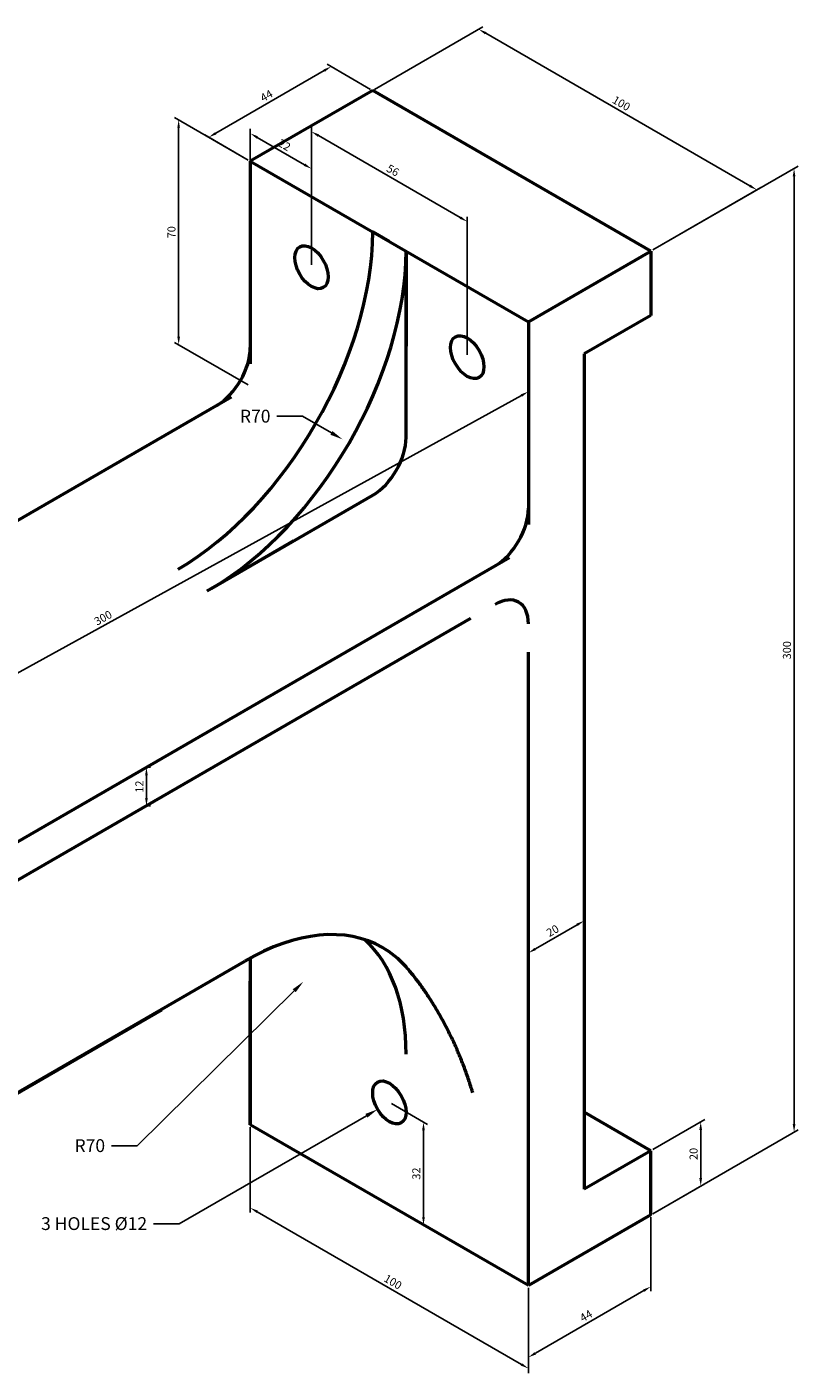
# Model space of a CAD drawing. Units: millimetres. Extents: x 3560 to 4017, y 1013 to 1432.
# Tile 2 of 2: x 3777 to 4017, y 1013 to 1432. Entities that reach past the tile are written whole.
import ezdxf
from ezdxf import colors
from ezdxf.entities.mleader import LeaderData, LeaderLine
from ezdxf.math import Vec2, Vec3

# ---------------------------------------------------------------- set-up
doc = ezdxf.new("R2010")
doc.units = ezdxf.units.MM
for name, color, linetype, lineweight in [('M-DIMS', 2, 'Continuous', 25), ('M-OUTL', 7, 'Continuous', 50), ('M-TEXT', 3, 'Continuous', 25)]:
    doc.layers.add(name, color=color, linetype=linetype, lineweight=lineweight)
doc.styles.get("Standard").update_dxf_attribs({"font": 'arial.ttf'})
doc.dimstyles.new('ISO-25', dxfattribs={"dimtxt": 2.5, "dimasz": 2.5, "dimexe": 1.25, "dimexo": 0.625, "dimtad": 1, "dimtxsty": 'Standard', "dimcen": 2.5, "dimadec": 0, "dimazin": 0, "dimtfac": 1, "dimtmove": 0, "dimatfit": 3, "dimfxl": 1, "dimarcsym": 0})

# ---------------------------------------------------------------- blocks, each defined once
blk = doc.blocks.new('*D1')
at = {"layer": 'Defpoints', "color": 0, "transparency": 16777216}
for p in [(3971.36, 1362.62), (4016, 1088.39), (3971.36, 1062.62)]:
    blk.add_point(p, dxfattribs=at)
at = {"layer": 'M-DIMS', "color": 0, "lineweight": -2, "transparency": 16777216}
for p, q in [((3971.99, 1362.99), (4017.25, 1389.12)), ((4016, 1385.89), (4016, 1090.89)), ((3971.99, 1062.99), (4017.25, 1089.12))]:
    blk.add_line(p, q, dxfattribs=at)
at = {"layer": 'M-DIMS', "color": 0, "transparency": 16777216}
for points in [[(4015.58, 1385.89), (4016.41, 1385.89), (4016, 1388.39)], [(4015.58, 1090.89), (4016.41, 1090.89), (4016, 1088.39)]]:
    blk.add_solid(points, dxfattribs=at)
at = {"layer": 'M-DIMS', "color": 0, "transparency": 16777216, "insert": (4014.09, 1238.39), "char_height": 2.5, "attachment_point": 5, "rotation": 90}
blk.add_mtext('300', dxfattribs=at)
blk = doc.blocks.new('*D2')
at = {"layer": 'Defpoints', "color": 0, "transparency": 16777216}
for p in [(3971.36, 1082.62), (3986.92, 1071.61), (3971.36, 1062.62)]:
    blk.add_point(p, dxfattribs=at)
at = {"layer": 'M-DIMS', "color": 0, "lineweight": -2, "transparency": 16777216}
for p, q in [((3971.99, 1082.99), (3988.17, 1092.33)), ((3986.92, 1089.11), (3986.92, 1074.11)), ((3971.99, 1062.99), (3988.17, 1072.33))]:
    blk.add_line(p, q, dxfattribs=at)
at = {"layer": 'M-DIMS', "color": 0, "transparency": 16777216}
for points in [[(3986.5, 1089.11), (3987.34, 1089.11), (3986.92, 1091.61)], [(3986.5, 1074.11), (3987.34, 1074.11), (3986.92, 1071.61)]]:
    blk.add_solid(points, dxfattribs=at)
at = {"layer": 'M-DIMS', "color": 0, "transparency": 16777216, "insert": (3985.02, 1081.61), "char_height": 2.5, "attachment_point": 5, "rotation": 90}
blk.add_mtext('20', dxfattribs=at)
blk = doc.blocks.new('*D3')
at = {"layer": 'Defpoints', "color": 0, "transparency": 16777216}
for p in [(3971.36, 1062.62), (3933.26, 1040.62), (3971.36, 1040.31)]:
    blk.add_point(p, dxfattribs=at)
at = {"layer": 'M-DIMS', "color": 0, "lineweight": -2, "transparency": 16777216}
for p, q in [((3971.36, 1061.9), (3971.36, 1038.87)), ((3933.26, 1039.9), (3933.26, 1016.87)), ((3935.42, 1019.56), (3969.2, 1039.06))]:
    blk.add_line(p, q, dxfattribs=at)
at = {"layer": 'M-DIMS', "color": 0, "transparency": 16777216}
for points in [[(3968.99, 1039.42), (3969.41, 1038.7), (3971.36, 1040.31)], [(3935.21, 1019.92), (3935.63, 1019.2), (3933.26, 1018.31)]]:
    blk.add_solid(points, dxfattribs=at)
at = {"layer": 'M-DIMS', "color": 0, "transparency": 16777216, "insert": (3951.37, 1030.94), "char_height": 2.5, "attachment_point": 5, "rotation": 30}
blk.add_mtext('44', dxfattribs=at)
blk = doc.blocks.new('*D4')
at = {"layer": 'Defpoints', "color": 0, "transparency": 16777216}
for p in [(3846.65, 1090.62), (3933.26, 1040.62), (3933.26, 1014.84)]:
    blk.add_point(p, dxfattribs=at)
at = {"layer": 'M-DIMS', "color": 0, "lineweight": -2, "transparency": 16777216}
for p, q in [((3846.65, 1089.9), (3846.65, 1063.4)), ((3848.82, 1063.59), (3931.09, 1016.09)), ((3933.26, 1039.9), (3933.26, 1013.4))]:
    blk.add_line(p, q, dxfattribs=at)
at = {"layer": 'M-DIMS', "color": 0, "transparency": 16777216}
for points in [[(3849.03, 1063.95), (3848.61, 1063.23), (3846.65, 1064.84)], [(3931.3, 1016.45), (3930.88, 1015.73), (3933.26, 1014.84)]]:
    blk.add_solid(points, dxfattribs=at)
at = {"layer": 'M-DIMS', "color": 0, "transparency": 16777216, "insert": (3890.91, 1041.49), "char_height": 2.5, "attachment_point": 5, "rotation": 330}
blk.add_mtext('100', dxfattribs=at)
blk = doc.blocks.new('*D5')
at = {"layer": 'Defpoints', "color": 0, "transparency": 16777216}
for p in [(3814.31, 1201.95), (3814.31, 1189.95), (3814.31, 1189.95)]:
    blk.add_point(p, dxfattribs=at)
at = {"layer": 'M-DIMS', "color": 0, "lineweight": -2, "transparency": 16777216}
for p, q in [((3814.31, 1199.45), (3814.31, 1192.45)), ((3814.93, 1201.95), (3815.56, 1201.95)), ((3814.93, 1189.95), (3815.56, 1189.95))]:
    blk.add_line(p, q, dxfattribs=at)
at = {"layer": 'M-DIMS', "color": 0, "transparency": 16777216}
for points in [[(3813.89, 1199.45), (3814.72, 1199.45), (3814.31, 1201.95)], [(3813.89, 1192.45), (3814.72, 1192.45), (3814.31, 1189.95)]]:
    blk.add_solid(points, dxfattribs=at)
at = {"layer": 'M-DIMS', "color": 0, "transparency": 16777216, "insert": (3812.43, 1195.95), "char_height": 2.5, "attachment_point": 5, "rotation": 90}
blk.add_mtext('12', dxfattribs=at)
blk = doc.blocks.new('*D6')
at = {"layer": 'Defpoints', "color": 0, "transparency": 16777216}
for p in [(3871.84, 1420.08), (3884.76, 1412.62), (3846.65, 1390.62)]:
    blk.add_point(p, dxfattribs=at)
at = {"layer": 'M-DIMS', "color": 0, "lineweight": -2, "transparency": 16777216}
for p, q in [((3884.13, 1412.99), (3870.59, 1420.8)), ((3835.9, 1399.33), (3869.68, 1418.83)), ((3846.03, 1390.99), (3832.49, 1398.8))]:
    blk.add_line(p, q, dxfattribs=at)
at = {"layer": 'M-DIMS', "color": 0, "transparency": 16777216}
for points in [[(3869.47, 1419.19), (3869.88, 1418.47), (3871.84, 1420.08)], [(3835.69, 1399.69), (3836.11, 1398.97), (3833.74, 1398.08)]]:
    blk.add_solid(points, dxfattribs=at)
at = {"layer": 'M-DIMS', "color": 0, "transparency": 16777216, "insert": (3851.85, 1410.71), "char_height": 2.5, "attachment_point": 5, "rotation": 30}
blk.add_mtext('44', dxfattribs=at)
blk = doc.blocks.new('*D7')
at = {"layer": 'Defpoints', "color": 0, "transparency": 16777216}
for p in [(3884.76, 1412.62), (4004.4, 1381.7), (3971.36, 1362.62)]:
    blk.add_point(p, dxfattribs=at)
at = {"layer": 'M-DIMS', "color": 0, "lineweight": -2, "transparency": 16777216}
for p, q in [((3885.38, 1412.99), (3919.04, 1432.42)), ((3919.96, 1430.45), (4002.23, 1382.95)), ((3971.99, 1362.99), (4005.65, 1382.42))]:
    blk.add_line(p, q, dxfattribs=at)
at = {"layer": 'M-DIMS', "color": 0, "transparency": 16777216}
for points in [[(3920.17, 1430.81), (3919.75, 1430.09), (3917.79, 1431.7)], [(4002.44, 1383.31), (4002.02, 1382.59), (4004.4, 1381.7)]]:
    blk.add_solid(points, dxfattribs=at)
at = {"layer": 'M-DIMS', "color": 0, "transparency": 16777216, "insert": (3962.05, 1408.34), "char_height": 2.5, "attachment_point": 5, "rotation": 330}
blk.add_mtext('100', dxfattribs=at)
blk = doc.blocks.new('*D8')
at = {"layer": 'Defpoints', "color": 0, "transparency": 16777216}
for p in [(3914.2, 1371.83), (3865.71, 1357.62), (3914.2, 1329.62)]:
    blk.add_point(p, dxfattribs=at)
at = {"layer": 'M-DIMS', "color": 0, "lineweight": -2, "transparency": 16777216}
for p, q in [((3865.71, 1358.35), (3865.71, 1401.27)), ((3867.87, 1398.58), (3912.04, 1373.08)), ((3914.2, 1330.35), (3914.2, 1373.27))]:
    blk.add_line(p, q, dxfattribs=at)
at = {"layer": 'M-DIMS', "color": 0, "transparency": 16777216}
for points in [[(3868.08, 1398.94), (3867.66, 1398.22), (3865.71, 1399.83)], [(3912.25, 1373.44), (3911.83, 1372.72), (3914.2, 1371.83)]]:
    blk.add_solid(points, dxfattribs=at)
at = {"layer": 'M-DIMS', "color": 0, "transparency": 16777216, "insert": (3890.91, 1387.48), "char_height": 2.5, "attachment_point": 5, "rotation": 330}
blk.add_mtext('56', dxfattribs=at)
blk = doc.blocks.new('*D9')
at = {"layer": 'Defpoints', "color": 0, "transparency": 16777216}
for p in [(3846.65, 1399.27), (3846.65, 1368.62), (3865.71, 1357.62)]:
    blk.add_point(p, dxfattribs=at)
at = {"layer": 'M-DIMS', "color": 0, "lineweight": -2, "transparency": 16777216}
for p, q in [((3846.65, 1369.35), (3846.65, 1400.71)), ((3863.54, 1389.52), (3848.82, 1398.02)), ((3865.71, 1358.35), (3865.71, 1389.71))]:
    blk.add_line(p, q, dxfattribs=at)
at = {"layer": 'M-DIMS', "color": 0, "transparency": 16777216}
for points in [[(3849.03, 1398.38), (3848.61, 1397.66), (3846.65, 1399.27)], [(3863.75, 1389.88), (3863.33, 1389.16), (3865.71, 1388.27)]]:
    blk.add_solid(points, dxfattribs=at)
at = {"layer": 'M-DIMS', "color": 0, "transparency": 16777216, "insert": (3857.12, 1395.39), "char_height": 2.5, "attachment_point": 5, "rotation": 330}
blk.add_mtext('22', dxfattribs=at)
blk = doc.blocks.new('*D10')
at = {"layer": 'Defpoints', "color": 0, "transparency": 16777216}
for p in [(3846.65, 1390.62), (3824.34, 1333.51), (3846.65, 1320.62)]:
    blk.add_point(p, dxfattribs=at)
at = {"layer": 'M-DIMS', "color": 0, "lineweight": -2, "transparency": 16777216}
for p, q in [((3846.03, 1390.99), (3823.09, 1404.23)), ((3824.34, 1401.01), (3824.34, 1336.01)), ((3846.03, 1320.99), (3823.09, 1334.23))]:
    blk.add_line(p, q, dxfattribs=at)
at = {"layer": 'M-DIMS', "color": 0, "transparency": 16777216}
for points in [[(3823.92, 1401.01), (3824.75, 1401.01), (3824.34, 1403.51)], [(3823.92, 1336.01), (3824.75, 1336.01), (3824.34, 1333.51)]]:
    blk.add_solid(points, dxfattribs=at)
at = {"layer": 'M-DIMS', "color": 0, "transparency": 16777216, "insert": (3822.43, 1368.51), "char_height": 2.5, "attachment_point": 5, "rotation": 90}
blk.add_mtext('70', dxfattribs=at)
blk = doc.blocks.new('*D11')
at = {"layer": 'Defpoints', "color": 0, "transparency": 16777216}
for p in [(3933.26, 1309.09), (3670.47, 1174.18), (3670.47, 1164.38)]:
    blk.add_point(p, dxfattribs=at)
at = {"layer": 'M-DIMS', "color": 0, "lineweight": -2, "transparency": 16777216}
for p, q in [((3933.26, 1309.8), (3933.26, 1320.32)), ((3931.07, 1317.69), (3672.66, 1175.38)), ((3670.47, 1165.09), (3670.47, 1175.61))]:
    blk.add_line(p, q, dxfattribs=at)
at = {"layer": 'M-DIMS', "color": 0, "transparency": 16777216}
for points in [[(3930.87, 1318.05), (3931.27, 1317.32), (3933.26, 1318.89)], [(3672.46, 1175.75), (3672.86, 1175.02), (3670.47, 1174.18)]]:
    blk.add_solid(points, dxfattribs=at)
at = {"layer": 'M-DIMS', "color": 0, "transparency": 16777216, "insert": (3800.95, 1248.2), "char_height": 2.5, "attachment_point": 5, "rotation": 28.8409}
blk.add_mtext('300', dxfattribs=at)
blk = doc.blocks.new('*D12')
at = {"layer": 'Defpoints', "color": 0, "transparency": 16777216}
for p in [(3889.96, 1097.62), (3889.96, 1065.62), (3900.59, 1059.49)]:
    blk.add_point(p, dxfattribs=at)
at = {"layer": 'M-DIMS', "color": 0, "lineweight": -2, "transparency": 16777216}
for p, q in [((3890.58, 1097.26), (3901.84, 1090.77)), ((3900.59, 1088.99), (3900.59, 1061.99)), ((3890.58, 1065.26), (3901.84, 1058.77))]:
    blk.add_line(p, q, dxfattribs=at)
at = {"layer": 'M-DIMS', "color": 0, "transparency": 16777216}
for points in [[(3900.17, 1088.99), (3901, 1088.99), (3900.59, 1091.49)], [(3900.17, 1061.99), (3901, 1061.99), (3900.59, 1059.49)]]:
    blk.add_solid(points, dxfattribs=at)
at = {"layer": 'M-DIMS', "color": 0, "transparency": 16777216, "insert": (3898.68, 1075.49), "char_height": 2.5, "attachment_point": 5, "rotation": 90}
blk.add_mtext('32', dxfattribs=at)
blk = doc.blocks.new('*D13')
at = {"layer": 'Defpoints', "color": 0, "transparency": 16777216}
for p in [(3950.58, 1154.17), (3950.58, 1149.23), (3933.26, 1139.23)]:
    blk.add_point(p, dxfattribs=at)
at = {"layer": 'M-DIMS', "color": 0, "lineweight": -2, "transparency": 16777216}
for p, q in [((3935.42, 1145.42), (3948.41, 1152.92)), ((3950.58, 1149.95), (3950.58, 1155.62)), ((3933.26, 1139.95), (3933.26, 1145.62))]:
    blk.add_line(p, q, dxfattribs=at)
at = {"layer": 'M-DIMS', "color": 0, "transparency": 16777216}
for points in [[(3948.2, 1153.28), (3948.62, 1152.56), (3950.58, 1154.17)], [(3935.21, 1145.78), (3935.63, 1145.06), (3933.26, 1144.17)]]:
    blk.add_solid(points, dxfattribs=at)
at = {"layer": 'M-DIMS', "color": 0, "transparency": 16777216, "insert": (3940.97, 1150.82), "char_height": 2.5, "attachment_point": 5, "rotation": 30}
blk.add_mtext('20', dxfattribs=at)

msp = doc.modelspace()

# ---------------------------------------------------------------- linework, layer by layer
at = {"layer": 'M-OUTL'}
for p, q in [((3884.76, 1412.625), (3846.655, 1390.625)), ((3971.362, 1362.625), (3884.76, 1412.625)), ((3846.655, 1390.625), (3933.257, 1340.625)), ((3846.655, 1390.625), (3846.655, 1327.553)), ((3889.956, 1365.625), (3884.76, 1368.625)), ((3895.152, 1362.625), (3895.152, 1333.039)), ((3895.154, 1304.625), (3895.154, 1362.625)), ((3933.257, 1340.625), (3971.362, 1362.625)), ((3971.362, 1362.625), (3971.362, 1342.625)), ((3971.362, 1362.625), (3971.362, 1342.625)), ((3971.362, 1342.625), (3950.578, 1330.625)), ((3933.257, 1340.625), (3933.257, 1277.553)), ((3950.578, 1330.625), (3950.578, 1070.625)), ((3840.655, 1317.16), (3656.796, 1211.009)), ((3834.532, 1257.625), (3884.762, 1286.625)), ((3860.152, 1272.417), (3833.104, 1256.801)), ((3927.257, 1267.16), (3691.45, 1131.017)), ((3915.257, 1248.232), (3681.057, 1113.017)), ((3933.257, 1040.625), (3933.257, 1237.84)), ((3668.255, 1039.625), (3844.925, 1141.625)), ((3846.657, 1142.596), (3846.657, 1090.625)), ((3846.655, 1090.625), (3846.655, 1135.416)), ((3711.991, 1064.578), (3819.138, 1126.439)), ((3971.364, 1082.625), (3950.58, 1094.625)), ((3933.257, 1040.625), (3846.655, 1090.625)), ((3971.362, 1082.625), (3950.578, 1070.625)), ((3971.362, 1062.625), (3971.362, 1082.625)), ((3971.362, 1062.625), (3933.257, 1040.625))]:
    msp.add_line(p, q, dxfattribs=at)
msp.add_lwpolyline([(3915.939, 1100.625), (3915.842, 1100.951), (3915.72, 1101.35), (3915.626, 1101.658), (3915.484, 1102.119), (3915.328, 1102.614), (3915.171, 1103.107), (3915.011, 1103.599), (3914.85, 1104.089), (3914.686, 1104.579), (3914.521, 1105.066), (3914.353, 1105.553), (3914.184, 1106.038), (3914.013, 1106.522), (3913.839, 1107.005), (3913.664, 1107.486), (3913.487, 1107.966), (3913.308, 1108.445), (3913.128, 1108.922), (3912.945, 1109.398), (3912.761, 1109.872), (3912.575, 1110.345), (3912.387, 1110.817), (3912.197, 1111.287), (3912.006, 1111.755), (3911.813, 1112.223), (3911.618, 1112.688), (3911.421, 1113.152), (3911.223, 1113.615), (3911.023, 1114.076), (3910.821, 1114.536), (3910.618, 1114.994), (3910.413, 1115.45), (3910.206, 1115.905), (3909.998, 1116.358), (3909.788, 1116.809), (3909.577, 1117.259), (3909.364, 1117.707), (3909.15, 1118.153), (3908.934, 1118.598), (3908.717, 1119.041), (3908.498, 1119.481), (3908.278, 1119.92), (3908.057, 1120.357), (3907.834, 1120.792), (3907.61, 1121.225), (3907.385, 1121.656), (3907.158, 1122.084), (3906.93, 1122.511), (3906.701, 1122.936), (3906.471, 1123.359), (3906.239, 1123.78), (3906.006, 1124.198), (3905.772, 1124.615), (3905.536, 1125.029), (3905.3, 1125.442), (3905.062, 1125.852), (3904.823, 1126.26), (3904.583, 1126.666), (3904.342, 1127.07), (3904.1, 1127.471), (3903.856, 1127.87), (3903.612, 1128.266), (3903.367, 1128.66), (3903.121, 1129.052), (3902.874, 1129.441), (3902.626, 1129.827), (3902.378, 1130.211), (3902.129, 1130.592), (3901.879, 1130.97), (3901.628, 1131.346), (3901.377, 1131.718), (3901.126, 1132.087), (3900.874, 1132.453), (3900.622, 1132.816), (3900.369, 1133.176), (3900.116, 1133.532), (3899.863, 1133.885), (3899.61, 1134.235), (3899.357, 1134.58), (3899.105, 1134.922), (3898.852, 1135.26), (3898.6, 1135.595), (3898.348, 1135.925), (3898.096, 1136.252), (3897.845, 1136.574), (3897.594, 1136.893), (3897.345, 1137.207), (3897.096, 1137.516), (3896.848, 1137.821), (3896.601, 1138.121), (3896.355, 1138.417), (3896.111, 1138.707), (3895.869, 1138.993), (3895.629, 1139.272), (3895.39, 1139.547), (3895.154, 1139.816)], dxfattribs=at)
for centre, major_axis, start_param, end_param in [((3824.138, 1333.626), (42.867, 74.248), 3.927014, 5.497764), ((3834.531, 1327.626), (42.867, 74.248), 3.927014, 5.497764), ((3836.264, 1326.625), (-7.348, -12.728), 0.7853982, 2.3561945), ((3884.762, 1298.625), (-7.348, -12.728), 0.7853982, 2.3561945), ((3922.867, 1276.625), (-7.348, -12.728), 0.7853982, 2.3561945), ((3922.867, 1240.625), (-7.348, -12.728), 3.1415927, 3.9269908), ((3922.867, 1240.625), (-7.348, -12.728), 2.3561945, 3.1415927), ((3844.923, 1071.623), (42.867, 74.248), 0, 0.785375), ((3834.531, 1077.623), (42.867, 74.248), 5.4978103, 6.161671), ((3844.923, 1071.623), (42.867, 74.248), 6.0920251, 6.2831853)]:
    msp.add_ellipse(centre, major_axis=major_axis, ratio=0.5773503, start_param=start_param, end_param=end_param, dxfattribs=at)
for centre in [(3865.707, 1357.625), (3914.205, 1329.625), (3889.956, 1097.625)]:
    msp.add_ellipse(centre, major_axis=(3.674, -6.364), ratio=0.5773503, dxfattribs=at)

# ---------------------------------------------------------------- dimensions: what is measured, and where the dimension line sits
at = {"layer": 'M-DIMS'}
for p1, p2, distance, picture, middle in [((3884.76, 1412.625), (3971.362, 1362.625), 33.033, '*D7', (3962.045, 1408.343)), ((3846.655, 1390.625), (3884.76, 1412.625), 12.919, '*D6', (3851.851, 1410.707)), ((3846.655, 1390.625), (3846.655, 1320.625), -22.32, '*D10', (3822.434, 1368.511)), ((3865.707, 1357.625), (3846.655, 1368.625), -26.536, '*D9', (3857.121, 1395.394)), ((3865.707, 1357.625), (3914.205, 1329.625), 36.551, '*D8', (3890.907, 1387.477)), ((3971.362, 1362.625), (3971.362, 1062.625), 44.635, '*D1', (4014.095, 1238.395)), ((3933.257, 1309.089), (3670.468, 1164.375), -8.588, '*D11', (3800.945, 1248.202)), ((3814.307, 1201.949), (3814.307, 1189.949), 0, '*D5', (3812.427, 1195.949)), ((3933.257, 1139.232), (3950.578, 1149.232), 4.278, '*D13', (3940.967, 1150.819)), ((3889.956, 1097.625), (3889.956, 1065.625), 10.63, '*D12', (3898.683, 1075.487)), ((3846.655, 1090.625), (3933.257, 1040.625), -22.329, '*D4', (3890.907, 1041.488)), ((3971.362, 1082.625), (3971.362, 1062.625), 15.559, '*D2', (3985.02, 1081.607)), ((3933.257, 1040.625), (3971.362, 1062.625), -19.322, '*D3', (3951.372, 1030.937))]:
    dim = msp.add_aligned_dim(p1=p1, p2=p2, distance=distance, dimstyle='ISO-25', override={"dimclrd": 0, "dimclre": 0, "dimclrt": 0}, dxfattribs=at)
    dim.commit()
    dim.dimension.update_dxf_attribs({"geometry": picture, "text_midpoint": middle})

# ---------------------------------------------------------------- leaders
at = {"layer": 'M-TEXT'}
ml = msp.add_multileader_mtext('Standard', dxfattribs=at)
ml.set_content('R70', color=256)
ml.set_leader_properties()
ml.build(insert=Vec2(0, 0))
ctx = ml.context
ctx.base_point, ctx.plane_origin = Vec3(3841.394, 1311.223), Vec3(3875.382, 1304.039)
ctx.text_align_type = 2
notes = []
notes.append((ctx, [(0, (1, 1, 0), (3862.938, 1311.223), (-1, 0), 8, [(0, [(3875.382, 1304.039)], 0, [])])]))
ctx.mtext.insert, ctx.mtext.alignment, ctx.mtext.flow_direction = Vec3(3852.938, 1313.258), 3, 5
ml = msp.add_multileader_mtext('Standard', dxfattribs=at)
ml.set_content('R70', color=256)
ml.set_leader_properties()
ml.build(insert=Vec2(0, 0))
ctx = ml.context
ctx.base_point, ctx.plane_origin = Vec3(3789.884, 1084.159), Vec3(3863.186, 1135.23)
ctx.text_align_type = 2
notes.append((ctx, [(0, (1, 1, 0), (3811.429, 1084.159), (-1, 0), 8, [(0, [(3863.186, 1135.23)], 0, [])])]))
ctx.mtext.insert, ctx.mtext.alignment, ctx.mtext.flow_direction = Vec3(3801.429, 1086.193), 3, 5
ml = msp.add_multileader_mtext('Standard', dxfattribs=at)
ml.set_content('3 HOLES %%C12', color=256)
ml.set_leader_properties()
ml.build(insert=Vec2(0, 0))
ctx = ml.context
ctx.base_point, ctx.plane_origin = Vec3(3777.332, 1059.846), Vec3(3886.282, 1095.503)
ctx.text_align_type = 2
notes.append((ctx, [(0, (1, 1, 0), (3824.522, 1059.846), (-1, 0), 8, [(0, [(3886.282, 1095.503)], 0, [])])]))
ctx.mtext.insert, ctx.mtext.alignment, ctx.mtext.flow_direction = Vec3(3814.522, 1061.927), 3, 5
for ctx, leaders in notes:
    for number, flags, end, landing, length, lines in leaders:
        leader = LeaderData()
        leader.index, (leader.has_last_leader_line, leader.has_dogleg_vector, leader.attachment_direction) = number, flags
        leader.last_leader_point, leader.dogleg_vector, leader.dogleg_length = Vec3(end), Vec3(landing), length
        for number, points, colour, breaks in lines:
            line = LeaderLine()
            line.index, line.vertices, line.color, line.breaks = number, Vec3.list(points), colors.encode_raw_color(colour), breaks
            leader.lines.append(line)
        ctx.leaders.append(leader)

doc.saveas('drawing.dxf')
